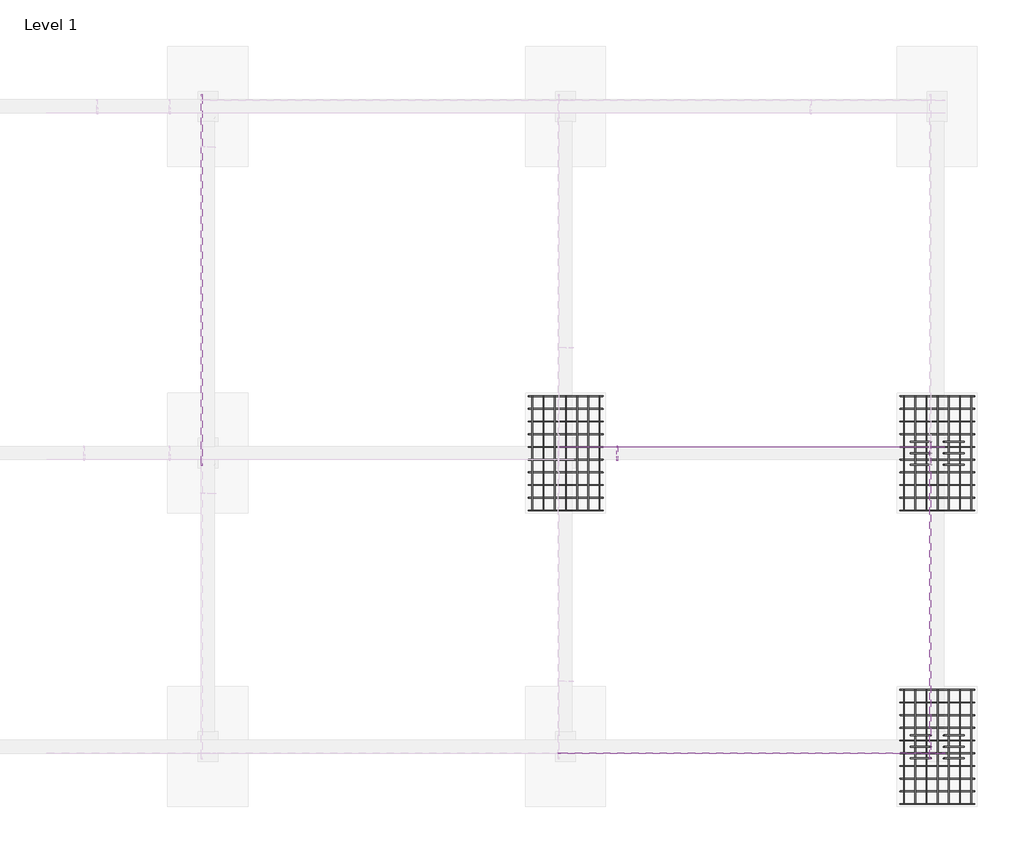
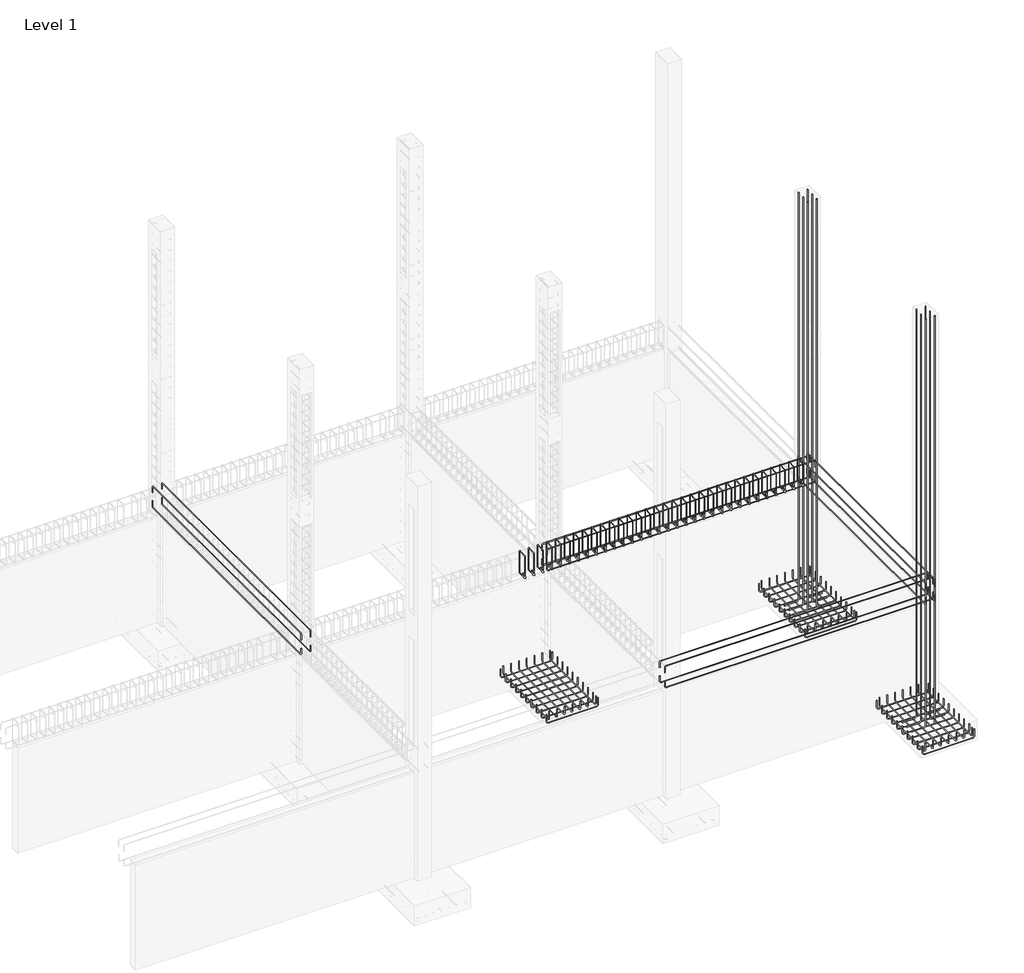
# One storey, part 6 of 8: 19 reinforcing bars.
"""IFC4 building model written with IfcOpenShell, lengths in millimetres."""

from ifc_helpers import new_model, si_unit, point, frame, origin, place, context, project, spatial, polyline, circle_curve, trimmed, segment, composite_curve, source, transform, mapped, element, save
from ifc_brep_helpers import swept_disk

model = new_model("IFC4")

# Units and contexts
model_context = context("Model", 3, world=origin())
ifc_project = project(units=[si_unit("LENGTHUNIT", "METRE", prefix="MILLI")], contexts=[model_context])

# Site, building, storey
site = spatial("IfcSite", under=ifc_project)
building = spatial("IfcBuilding", under=site)
storey = spatial("IfcBuildingStorey", under=building, Name="Level 1", Elevation=0.0)

# Reinforcing bars
placement = place(None, origin())
reinforcing_bar_shape = source(origin(), model_context, "Body", "SolidModel", [
    swept_disk(composite_curve([segment(polyline([(-3147.528716, 3219.1306965, 2643.0183362), (-3147.528716, 3219.1306965, 2528.7183362)]), True, "CONTINUOUS"), segment(trimmed(circle_curve(frame((-3182.072716, 3219.1306965, 2528.7183362), z_axis=(0.0, 1.0, 0.0), x_axis=(34.544000000000324, 0.0, 0.0)), 34.544), [point((-3147.528716, 3219.1306965, 2528.7183362))], [point((-3182.072716, 3219.1306965, 2494.1743362))], True, "CARTESIAN"), True, "CONTINUOUS"), segment(polyline([(-3182.072716, 3219.1306965, 2494.1743362), (-8989.4602157, 3219.1306965, 2494.1743362)]), True, "CONTINUOUS"), segment(trimmed(circle_curve(frame((-8989.4602157, 3219.1306965, 2528.7183362), z_axis=(0.0, 1.0, 0.0), x_axis=(0.0, 0.0, -34.54399999999987)), 34.544), [point((-8989.4602157, 3219.1306965, 2494.1743362))], [point((-9024.0042157, 3219.1306965, 2528.7183362))], True, "CARTESIAN"), True, "CONTINUOUS"), segment(polyline([(-9024.0042157, 3219.1306965, 2528.7183362), (-9024.0042157, 3219.1306965, 2643.0183362)]), True, "CONTINUOUS")], self_intersect=False), 5.969),
])
element("IfcReinforcingBar", 1, at=placement, inside=storey, context=model_context, shape_type="MappedRepresentation", body=[
    mapped(reinforcing_bar_shape, transform((0.0, 0.0, 0.0), x_axis=(1.0, 0.0, 0.0), y_axis=(0.0, 1.0, 0.0), z_axis=(0.0, 0.0, 1.0))),
    mapped(reinforcing_bar_shape, transform((0.0, -193.2513276, 0.0), x_axis=(1.0, 0.0, 0.0), y_axis=(0.0, 1.0, 0.0), z_axis=(0.0, 0.0, 1.0))),
])
reinforcing_bar_2_shape = source(origin(), model_context, "Body", "SolidModel", [
    swept_disk(composite_curve([segment(polyline([(-9024.0042157, 3219.1306965, 2843.3816638), (-9024.0042157, 3219.1306965, 2957.6816638)]), True, "CONTINUOUS"), segment(trimmed(circle_curve(frame((-8989.4602157, 3219.1306965, 2957.6816638), z_axis=(0.0, 1.0, 0.0), x_axis=(-34.54399999999987, 0.0, 0.0)), 34.544), [point((-9024.0042157, 3219.1306965, 2957.6816638))], [point((-8989.4602157, 3219.1306965, 2992.2256638))], True, "CARTESIAN"), True, "CONTINUOUS"), segment(polyline([(-8989.4602157, 3219.1306965, 2992.2256638), (-3182.072716, 3219.1306965, 2992.2256638)]), True, "CONTINUOUS"), segment(trimmed(circle_curve(frame((-3182.072716, 3219.1306965, 2957.6816638), z_axis=(0.0, 1.0, 0.0), x_axis=(0.0, 0.0, 34.54399999999987)), 34.544), [point((-3182.072716, 3219.1306965, 2992.2256638))], [point((-3147.528716, 3219.1306965, 2957.6816638))], True, "CARTESIAN"), True, "CONTINUOUS"), segment(polyline([(-3147.528716, 3219.1306965, 2957.6816638), (-3147.528716, 3219.1306965, 2843.3816638)]), True, "CONTINUOUS")], self_intersect=False), 5.969),
])
element("IfcReinforcingBar", 2, at=placement, inside=storey, context=model_context, shape_type="MappedRepresentation", body=[
    mapped(reinforcing_bar_2_shape, transform((0.0, 0.0, 0.0), x_axis=(1.0, 0.0, 0.0), y_axis=(0.0, 1.0, 0.0), z_axis=(0.0, 0.0, 1.0))),
    mapped(reinforcing_bar_2_shape, transform((0.0, -193.2513276, 0.0), x_axis=(1.0, 0.0, 0.0), y_axis=(0.0, 1.0, 0.0), z_axis=(0.0, 0.0, 1.0))),
])
reinforcing_bar_3_shape = source(origin(), model_context, "Body", "SolidModel", [
    swept_disk(composite_curve([segment(polyline([(-3157.434716, 7767.9070829, 9105.9), (-3157.434716, 7767.9070829, -307.9115)]), True, "CONTINUOUS"), segment(trimmed(circle_curve(frame((-3111.333716, 7767.9070829, -307.9115), z_axis=(0.0, -1.0, 0.0), x_axis=(-46.10100000000011, 0.0, 0.0)), 46.101), [point((-3157.434716, 7767.9070829, -307.9115))], [point((-3111.333716, 7767.9070829, -354.0125))], True, "CARTESIAN"), True, "CONTINUOUS"), segment(polyline([(-3111.333716, 7767.9070829, -354.0125), (-2844.760716, 7767.9070829, -354.0125)]), True, "CONTINUOUS")], self_intersect=False), 8.001),
])
element("IfcReinforcingBar", 3, at=placement, inside=storey, context=model_context, shape_type="MappedRepresentation", body=[
    mapped(reinforcing_bar_3_shape, transform((0.0, 0.0, 0.0), x_axis=(1.0, 0.0, 0.0), y_axis=(0.0, 1.0, 0.0), z_axis=(0.0, 0.0, 1.0))),
    mapped(reinforcing_bar_3_shape, transform((0.0, -174.625, 0.0), x_axis=(1.0, 0.0, 0.0), y_axis=(0.0, 1.0, 0.0), z_axis=(0.0, 0.0, 1.0))),
    mapped(reinforcing_bar_3_shape, transform((0.0, -349.25, 0.0), x_axis=(1.0, 0.0, 0.0), y_axis=(0.0, 1.0, 0.0), z_axis=(0.0, 0.0, 1.0))),
])
reinforcing_bar_4_shape = source(origin(), model_context, "Body", "SolidModel", [
    swept_disk(composite_curve([segment(polyline([(-3666.958716, 7767.9070829, -354.0125), (-3400.385716, 7767.9070829, -354.0125)]), True, "CONTINUOUS"), segment(trimmed(circle_curve(frame((-3400.385716, 7767.9070829, -307.9115), z_axis=(0.0, -1.0, 0.0), x_axis=(0.0, 0.0, -46.101)), 46.101), [point((-3400.385716, 7767.9070829, -354.0125))], [point((-3354.284716, 7767.9070829, -307.9115))], True, "CARTESIAN"), True, "CONTINUOUS"), segment(polyline([(-3354.284716, 7767.9070829, -307.9115), (-3354.284716, 7767.9070829, 9105.9)]), True, "CONTINUOUS")], self_intersect=False), 8.001),
])
element("IfcReinforcingBar", 4, at=placement, inside=storey, context=model_context, shape_type="MappedRepresentation", body=[
    mapped(reinforcing_bar_4_shape, transform((0.0, 0.0, 0.0), x_axis=(1.0, 0.0, 0.0), y_axis=(0.0, 1.0, 0.0), z_axis=(0.0, 0.0, 1.0))),
    mapped(reinforcing_bar_4_shape, transform((0.0, -174.625, 0.0), x_axis=(1.0, 0.0, 0.0), y_axis=(0.0, 1.0, 0.0), z_axis=(0.0, 0.0, 1.0))),
    mapped(reinforcing_bar_4_shape, transform((0.0, -349.25, 0.0), x_axis=(1.0, 0.0, 0.0), y_axis=(0.0, 1.0, 0.0), z_axis=(0.0, 0.0, 1.0))),
])
reinforcing_bar_5_shape = source(origin(), model_context, "Body", "SolidModel", [
    swept_disk(composite_curve([segment(polyline([(-3157.434716, 3297.1300327, 9105.9), (-3157.434716, 3297.1300327, -307.9115)]), True, "CONTINUOUS"), segment(trimmed(circle_curve(frame((-3111.333716, 3297.1300327, -307.9115), z_axis=(0.0, -1.0, 0.0), x_axis=(-46.10100000000011, 0.0, 0.0)), 46.101), [point((-3157.434716, 3297.1300327, -307.9115))], [point((-3111.333716, 3297.1300327, -354.0125))], True, "CARTESIAN"), True, "CONTINUOUS"), segment(polyline([(-3111.333716, 3297.1300327, -354.0125), (-2844.760716, 3297.1300327, -354.0125)]), True, "CONTINUOUS")], self_intersect=False), 8.001),
])
element("IfcReinforcingBar", 5, at=placement, inside=storey, context=model_context, shape_type="MappedRepresentation", body=[
    mapped(reinforcing_bar_5_shape, transform((0.0, 0.0, 0.0), x_axis=(1.0, 0.0, 0.0), y_axis=(0.0, 1.0, 0.0), z_axis=(0.0, 0.0, 1.0))),
    mapped(reinforcing_bar_5_shape, transform((0.0, -174.625, 0.0), x_axis=(1.0, 0.0, 0.0), y_axis=(0.0, 1.0, 0.0), z_axis=(0.0, 0.0, 1.0))),
    mapped(reinforcing_bar_5_shape, transform((0.0, -349.25, 0.0), x_axis=(1.0, 0.0, 0.0), y_axis=(0.0, 1.0, 0.0), z_axis=(0.0, 0.0, 1.0))),
])
reinforcing_bar_6_shape = source(origin(), model_context, "Body", "SolidModel", [
    swept_disk(composite_curve([segment(polyline([(-3666.958716, 3297.1300327, -354.0125), (-3400.385716, 3297.1300327, -354.0125)]), True, "CONTINUOUS"), segment(trimmed(circle_curve(frame((-3400.385716, 3297.1300327, -307.9115), z_axis=(0.0, -1.0, 0.0), x_axis=(0.0, 0.0, -46.101)), 46.101), [point((-3400.385716, 3297.1300327, -354.0125))], [point((-3354.284716, 3297.1300327, -307.9115))], True, "CARTESIAN"), True, "CONTINUOUS"), segment(polyline([(-3354.284716, 3297.1300327, -307.9115), (-3354.284716, 3297.1300327, 9105.9)]), True, "CONTINUOUS")], self_intersect=False), 8.001),
])
element("IfcReinforcingBar", 6, at=placement, inside=storey, context=model_context, shape_type="MappedRepresentation", body=[
    mapped(reinforcing_bar_6_shape, transform((0.0, 0.0, 0.0), x_axis=(1.0, 0.0, 0.0), y_axis=(0.0, 1.0, 0.0), z_axis=(0.0, 0.0, 1.0))),
    mapped(reinforcing_bar_6_shape, transform((0.0, -174.625, 0.0), x_axis=(1.0, 0.0, 0.0), y_axis=(0.0, 1.0, 0.0), z_axis=(0.0, 0.0, 1.0))),
    mapped(reinforcing_bar_6_shape, transform((0.0, -349.25, 0.0), x_axis=(1.0, 0.0, 0.0), y_axis=(0.0, 1.0, 0.0), z_axis=(0.0, 0.0, 1.0))),
])
reinforcing_bar_7_shape = source(origin(), model_context, "Body", "SolidModel", [
    swept_disk(composite_curve([segment(polyline([(-2690.328716, 8463.6130829, -216.662), (-2690.328716, 8463.6130829, -369.062)]), True, "CONTINUOUS"), segment(trimmed(circle_curve(frame((-2734.397716, 8463.6130829, -369.062), z_axis=(0.0, 1.0, 0.0), x_axis=(44.06899999999996, 0.0, 0.0)), 44.069), [point((-2690.328716, 8463.6130829, -369.062))], [point((-2734.397716, 8463.6130829, -413.131))], True, "CARTESIAN"), True, "CONTINUOUS"), segment(polyline([(-2734.397716, 8463.6130829, -413.131), (-3777.321716, 8463.6130829, -413.131)]), True, "CONTINUOUS"), segment(trimmed(circle_curve(frame((-3777.321716, 8463.6130829, -369.062), z_axis=(0.0, 1.0, 0.0), x_axis=(0.0, 0.0, -44.06899999999996)), 44.069), [point((-3777.321716, 8463.6130829, -413.131))], [point((-3821.390716, 8463.6130829, -369.062))], True, "CARTESIAN"), True, "CONTINUOUS"), segment(polyline([(-3821.390716, 8463.6130829, -369.062), (-3821.390716, 8463.6130829, -216.662)]), True, "CONTINUOUS")], self_intersect=False), 5.969),
])
element("IfcReinforcingBar", 7, at=placement, inside=storey, context=model_context, shape_type="MappedRepresentation", body=[
    mapped(reinforcing_bar_7_shape, transform((0.0, 0.0, 0.0), x_axis=(1.0, 0.0, 0.0), y_axis=(0.0, 1.0, 0.0), z_axis=(0.0, 0.0, 1.0))),
    mapped(reinforcing_bar_7_shape, transform((0.0, -193.4068889, 0.0), x_axis=(1.0, 0.0, 0.0), y_axis=(0.0, 1.0, 0.0), z_axis=(0.0, 0.0, 1.0))),
    mapped(reinforcing_bar_7_shape, transform((0.0, -386.8137778, 0.0), x_axis=(1.0, 0.0, 0.0), y_axis=(0.0, 1.0, 0.0), z_axis=(0.0, 0.0, 1.0))),
    mapped(reinforcing_bar_7_shape, transform((0.0, -580.2206667, 0.0), x_axis=(1.0, 0.0, 0.0), y_axis=(0.0, 1.0, 0.0), z_axis=(0.0, 0.0, 1.0))),
    mapped(reinforcing_bar_7_shape, transform((0.0, -773.6275556, 0.0), x_axis=(1.0, 0.0, 0.0), y_axis=(0.0, 1.0, 0.0), z_axis=(0.0, 0.0, 1.0))),
    mapped(reinforcing_bar_7_shape, transform((0.0, -967.0344444, 0.0), x_axis=(1.0, 0.0, 0.0), y_axis=(0.0, 1.0, 0.0), z_axis=(0.0, 0.0, 1.0))),
    mapped(reinforcing_bar_7_shape, transform((0.0, -1160.4413333, 0.0), x_axis=(1.0, 0.0, 0.0), y_axis=(0.0, 1.0, 0.0), z_axis=(0.0, 0.0, 1.0))),
    mapped(reinforcing_bar_7_shape, transform((0.0, -1353.8482222, 0.0), x_axis=(1.0, 0.0, 0.0), y_axis=(0.0, 1.0, 0.0), z_axis=(0.0, 0.0, 1.0))),
    mapped(reinforcing_bar_7_shape, transform((0.0, -1547.2551111, 0.0), x_axis=(1.0, 0.0, 0.0), y_axis=(0.0, 1.0, 0.0), z_axis=(0.0, 0.0, 1.0))),
    mapped(reinforcing_bar_7_shape, transform((0.0, -1740.662, 0.0), x_axis=(1.0, 0.0, 0.0), y_axis=(0.0, 1.0, 0.0), z_axis=(0.0, 0.0, 1.0))),
])
reinforcing_bar_8_shape = source(origin(), model_context, "Body", "SolidModel", [
    swept_disk(composite_curve([segment(polyline([(-3763.859716, 8463.6130829, -165.481), (-3763.859716, 8463.6130829, -317.881)]), True, "CONTINUOUS"), segment(trimmed(circle_curve(frame((-3763.859716, 8419.5440829, -317.881), z_axis=(-1.0, 0.0, 0.0), x_axis=(0.0, 44.068999999999505, 0.0)), 44.069), [point((-3763.859716, 8463.6130829, -317.881))], [point((-3763.859716, 8419.5440829, -361.95))], True, "CARTESIAN"), True, "CONTINUOUS"), segment(polyline([(-3763.859716, 8419.5440829, -361.95), (-3763.859716, 6767.0200829, -361.95)]), True, "CONTINUOUS"), segment(trimmed(circle_curve(frame((-3763.859716, 6767.0200829, -317.881), z_axis=(-1.0, 0.0, 0.0), x_axis=(0.0, 0.0, -44.06900000000002)), 44.069), [point((-3763.859716, 6767.0200829, -361.95))], [point((-3763.859716, 6722.9510829, -317.881))], True, "CARTESIAN"), True, "CONTINUOUS"), segment(polyline([(-3763.859716, 6722.9510829, -317.881), (-3763.859716, 6722.9510829, -165.481)]), True, "CONTINUOUS")], self_intersect=False), 5.969),
])
element("IfcReinforcingBar", 8, at=placement, inside=storey, context=model_context, shape_type="MappedRepresentation", body=[
    mapped(reinforcing_bar_8_shape, transform((0.0, 0.0, 0.0), x_axis=(1.0, 0.0, 0.0), y_axis=(0.0, 1.0, 0.0), z_axis=(0.0, 0.0, 1.0))),
    mapped(reinforcing_bar_8_shape, transform((170.5954914, 0.0, 0.0), x_axis=(1.0, 0.0, 0.0), y_axis=(0.0, 1.0, 0.0), z_axis=(0.0, 0.0, 1.0))),
    mapped(reinforcing_bar_8_shape, transform((341.1909829, 0.0, 0.0), x_axis=(1.0, 0.0, 0.0), y_axis=(0.0, 1.0, 0.0), z_axis=(0.0, 0.0, 1.0))),
    mapped(reinforcing_bar_8_shape, transform((511.7864743, 0.0, 0.0), x_axis=(1.0, 0.0, 0.0), y_axis=(0.0, 1.0, 0.0), z_axis=(0.0, 0.0, 1.0))),
    mapped(reinforcing_bar_8_shape, transform((682.3819658, 0.0, 0.0), x_axis=(1.0, 0.0, 0.0), y_axis=(0.0, 1.0, 0.0), z_axis=(0.0, 0.0, 1.0))),
    mapped(reinforcing_bar_8_shape, transform((852.9774572, 0.0, 0.0), x_axis=(1.0, 0.0, 0.0), y_axis=(0.0, 1.0, 0.0), z_axis=(0.0, 0.0, 1.0))),
    mapped(reinforcing_bar_8_shape, transform((1023.5729487, 0.0, 0.0), x_axis=(1.0, 0.0, 0.0), y_axis=(0.0, 1.0, 0.0), z_axis=(0.0, 0.0, 1.0))),
])
reinforcing_bar_9_shape = source(origin(), model_context, "Body", "SolidModel", [
    swept_disk(composite_curve([segment(polyline([(-8350.1422157, 8463.6130829, -216.662), (-8350.1422157, 8463.6130829, -369.062)]), True, "CONTINUOUS"), segment(trimmed(circle_curve(frame((-8394.2112157, 8463.6130829, -369.062), z_axis=(0.0, 1.0, 0.0), x_axis=(44.068999999999505, 0.0, 0.0)), 44.069), [point((-8350.1422157, 8463.6130829, -369.062))], [point((-8394.2112157, 8463.6130829, -413.131))], True, "CARTESIAN"), True, "CONTINUOUS"), segment(polyline([(-8394.2112157, 8463.6130829, -413.131), (-9437.1352157, 8463.6130829, -413.131)]), True, "CONTINUOUS"), segment(trimmed(circle_curve(frame((-9437.1352157, 8463.6130829, -369.062), z_axis=(0.0, 1.0, 0.0), x_axis=(0.0, 0.0, -44.06899999999996)), 44.069), [point((-9437.1352157, 8463.6130829, -413.131))], [point((-9481.2042157, 8463.6130829, -369.062))], True, "CARTESIAN"), True, "CONTINUOUS"), segment(polyline([(-9481.2042157, 8463.6130829, -369.062), (-9481.2042157, 8463.6130829, -216.662)]), True, "CONTINUOUS")], self_intersect=False), 5.969),
])
element("IfcReinforcingBar", 9, at=placement, inside=storey, context=model_context, shape_type="MappedRepresentation", body=[
    mapped(reinforcing_bar_9_shape, transform((0.0, 0.0, 0.0), x_axis=(1.0, 0.0, 0.0), y_axis=(0.0, 1.0, 0.0), z_axis=(0.0, 0.0, 1.0))),
    mapped(reinforcing_bar_9_shape, transform((0.0, -193.4068889, 0.0), x_axis=(1.0, 0.0, 0.0), y_axis=(0.0, 1.0, 0.0), z_axis=(0.0, 0.0, 1.0))),
    mapped(reinforcing_bar_9_shape, transform((0.0, -386.8137778, 0.0), x_axis=(1.0, 0.0, 0.0), y_axis=(0.0, 1.0, 0.0), z_axis=(0.0, 0.0, 1.0))),
    mapped(reinforcing_bar_9_shape, transform((0.0, -580.2206667, 0.0), x_axis=(1.0, 0.0, 0.0), y_axis=(0.0, 1.0, 0.0), z_axis=(0.0, 0.0, 1.0))),
    mapped(reinforcing_bar_9_shape, transform((0.0, -773.6275556, 0.0), x_axis=(1.0, 0.0, 0.0), y_axis=(0.0, 1.0, 0.0), z_axis=(0.0, 0.0, 1.0))),
    mapped(reinforcing_bar_9_shape, transform((0.0, -967.0344444, 0.0), x_axis=(1.0, 0.0, 0.0), y_axis=(0.0, 1.0, 0.0), z_axis=(0.0, 0.0, 1.0))),
    mapped(reinforcing_bar_9_shape, transform((0.0, -1160.4413333, 0.0), x_axis=(1.0, 0.0, 0.0), y_axis=(0.0, 1.0, 0.0), z_axis=(0.0, 0.0, 1.0))),
    mapped(reinforcing_bar_9_shape, transform((0.0, -1353.8482222, 0.0), x_axis=(1.0, 0.0, 0.0), y_axis=(0.0, 1.0, 0.0), z_axis=(0.0, 0.0, 1.0))),
    mapped(reinforcing_bar_9_shape, transform((0.0, -1547.2551111, 0.0), x_axis=(1.0, 0.0, 0.0), y_axis=(0.0, 1.0, 0.0), z_axis=(0.0, 0.0, 1.0))),
    mapped(reinforcing_bar_9_shape, transform((0.0, -1740.662, 0.0), x_axis=(1.0, 0.0, 0.0), y_axis=(0.0, 1.0, 0.0), z_axis=(0.0, 0.0, 1.0))),
])
reinforcing_bar_10_shape = source(origin(), model_context, "Body", "SolidModel", [
    swept_disk(composite_curve([segment(polyline([(-9423.6732157, 8463.6130829, -165.481), (-9423.6732157, 8463.6130829, -317.881)]), True, "CONTINUOUS"), segment(trimmed(circle_curve(frame((-9423.6732157, 8419.5440829, -317.881), z_axis=(-1.0, 0.0, 0.0), x_axis=(0.0, 44.068999999999505, 0.0)), 44.069), [point((-9423.6732157, 8463.6130829, -317.881))], [point((-9423.6732157, 8419.5440829, -361.95))], True, "CARTESIAN"), True, "CONTINUOUS"), segment(polyline([(-9423.6732157, 8419.5440829, -361.95), (-9423.6732157, 6767.0200829, -361.95)]), True, "CONTINUOUS"), segment(trimmed(circle_curve(frame((-9423.6732157, 6767.0200829, -317.881), z_axis=(-1.0, 0.0, 0.0), x_axis=(0.0, 0.0, -44.06900000000002)), 44.069), [point((-9423.6732157, 6767.0200829, -361.95))], [point((-9423.6732157, 6722.9510829, -317.881))], True, "CARTESIAN"), True, "CONTINUOUS"), segment(polyline([(-9423.6732157, 6722.9510829, -317.881), (-9423.6732157, 6722.9510829, -165.481)]), True, "CONTINUOUS")], self_intersect=False), 5.969),
])
element("IfcReinforcingBar", 10, at=placement, inside=storey, context=model_context, shape_type="MappedRepresentation", body=[
    mapped(reinforcing_bar_10_shape, transform((0.0, 0.0, 0.0), x_axis=(1.0, 0.0, 0.0), y_axis=(0.0, 1.0, 0.0), z_axis=(0.0, 0.0, 1.0))),
    mapped(reinforcing_bar_10_shape, transform((170.5954914, 0.0, 0.0), x_axis=(1.0, 0.0, 0.0), y_axis=(0.0, 1.0, 0.0), z_axis=(0.0, 0.0, 1.0))),
    mapped(reinforcing_bar_10_shape, transform((341.1909829, 0.0, 0.0), x_axis=(1.0, 0.0, 0.0), y_axis=(0.0, 1.0, 0.0), z_axis=(0.0, 0.0, 1.0))),
    mapped(reinforcing_bar_10_shape, transform((511.7864743, 0.0, 0.0), x_axis=(1.0, 0.0, 0.0), y_axis=(0.0, 1.0, 0.0), z_axis=(0.0, 0.0, 1.0))),
    mapped(reinforcing_bar_10_shape, transform((682.3819658, 0.0, 0.0), x_axis=(1.0, 0.0, 0.0), y_axis=(0.0, 1.0, 0.0), z_axis=(0.0, 0.0, 1.0))),
    mapped(reinforcing_bar_10_shape, transform((852.9774572, 0.0, 0.0), x_axis=(1.0, 0.0, 0.0), y_axis=(0.0, 1.0, 0.0), z_axis=(0.0, 0.0, 1.0))),
    mapped(reinforcing_bar_10_shape, transform((1023.5729487, 0.0, 0.0), x_axis=(1.0, 0.0, 0.0), y_axis=(0.0, 1.0, 0.0), z_axis=(0.0, 0.0, 1.0))),
])
reinforcing_bar_11_shape = source(origin(), model_context, "Body", "SolidModel", [
    swept_disk(composite_curve([segment(polyline([(-2690.328716, 3992.8360327, -216.662), (-2690.328716, 3992.8360327, -369.062)]), True, "CONTINUOUS"), segment(trimmed(circle_curve(frame((-2734.397716, 3992.8360327, -369.062), z_axis=(0.0, 1.0, 0.0), x_axis=(44.06899999999996, 0.0, 0.0)), 44.069), [point((-2690.328716, 3992.8360327, -369.062))], [point((-2734.397716, 3992.8360327, -413.131))], True, "CARTESIAN"), True, "CONTINUOUS"), segment(polyline([(-2734.397716, 3992.8360327, -413.131), (-3777.321716, 3992.8360327, -413.131)]), True, "CONTINUOUS"), segment(trimmed(circle_curve(frame((-3777.321716, 3992.8360327, -369.062), z_axis=(0.0, 1.0, 0.0), x_axis=(0.0, 0.0, -44.06899999999996)), 44.069), [point((-3777.321716, 3992.8360327, -413.131))], [point((-3821.390716, 3992.8360327, -369.062))], True, "CARTESIAN"), True, "CONTINUOUS"), segment(polyline([(-3821.390716, 3992.8360327, -369.062), (-3821.390716, 3992.8360327, -216.662)]), True, "CONTINUOUS")], self_intersect=False), 5.969),
])
element("IfcReinforcingBar", 11, at=placement, inside=storey, context=model_context, shape_type="MappedRepresentation", body=[
    mapped(reinforcing_bar_11_shape, transform((0.0, 0.0, 0.0), x_axis=(1.0, 0.0, 0.0), y_axis=(0.0, 1.0, 0.0), z_axis=(0.0, 0.0, 1.0))),
    mapped(reinforcing_bar_11_shape, transform((0.0, -193.4068889, 0.0), x_axis=(1.0, 0.0, 0.0), y_axis=(0.0, 1.0, 0.0), z_axis=(0.0, 0.0, 1.0))),
    mapped(reinforcing_bar_11_shape, transform((0.0, -386.8137778, 0.0), x_axis=(1.0, 0.0, 0.0), y_axis=(0.0, 1.0, 0.0), z_axis=(0.0, 0.0, 1.0))),
    mapped(reinforcing_bar_11_shape, transform((0.0, -580.2206667, 0.0), x_axis=(1.0, 0.0, 0.0), y_axis=(0.0, 1.0, 0.0), z_axis=(0.0, 0.0, 1.0))),
    mapped(reinforcing_bar_11_shape, transform((0.0, -773.6275556, 0.0), x_axis=(1.0, 0.0, 0.0), y_axis=(0.0, 1.0, 0.0), z_axis=(0.0, 0.0, 1.0))),
    mapped(reinforcing_bar_11_shape, transform((0.0, -967.0344444, 0.0), x_axis=(1.0, 0.0, 0.0), y_axis=(0.0, 1.0, 0.0), z_axis=(0.0, 0.0, 1.0))),
    mapped(reinforcing_bar_11_shape, transform((0.0, -1160.4413333, 0.0), x_axis=(1.0, 0.0, 0.0), y_axis=(0.0, 1.0, 0.0), z_axis=(0.0, 0.0, 1.0))),
    mapped(reinforcing_bar_11_shape, transform((0.0, -1353.8482222, 0.0), x_axis=(1.0, 0.0, 0.0), y_axis=(0.0, 1.0, 0.0), z_axis=(0.0, 0.0, 1.0))),
    mapped(reinforcing_bar_11_shape, transform((0.0, -1547.2551111, 0.0), x_axis=(1.0, 0.0, 0.0), y_axis=(0.0, 1.0, 0.0), z_axis=(0.0, 0.0, 1.0))),
    mapped(reinforcing_bar_11_shape, transform((0.0, -1740.662, 0.0), x_axis=(1.0, 0.0, 0.0), y_axis=(0.0, 1.0, 0.0), z_axis=(0.0, 0.0, 1.0))),
])
reinforcing_bar_12_shape = source(origin(), model_context, "Body", "SolidModel", [
    swept_disk(composite_curve([segment(polyline([(-3763.859716, 3992.8360327, -165.481), (-3763.859716, 3992.8360327, -317.881)]), True, "CONTINUOUS"), segment(trimmed(circle_curve(frame((-3763.859716, 3948.7670327, -317.881), z_axis=(-1.0, 0.0, 0.0), x_axis=(0.0, 44.06899999999996, 0.0)), 44.069), [point((-3763.859716, 3992.8360327, -317.881))], [point((-3763.859716, 3948.7670327, -361.95))], True, "CARTESIAN"), True, "CONTINUOUS"), segment(polyline([(-3763.859716, 3948.7670327, -361.95), (-3763.859716, 2296.2430327, -361.95)]), True, "CONTINUOUS"), segment(trimmed(circle_curve(frame((-3763.859716, 2296.2430327, -317.881), z_axis=(-1.0, 0.0, 0.0), x_axis=(0.0, 0.0, -44.06900000000002)), 44.069), [point((-3763.859716, 2296.2430327, -361.95))], [point((-3763.859716, 2252.1740327, -317.881))], True, "CARTESIAN"), True, "CONTINUOUS"), segment(polyline([(-3763.859716, 2252.1740327, -317.881), (-3763.859716, 2252.1740327, -165.481)]), True, "CONTINUOUS")], self_intersect=False), 5.969),
])
element("IfcReinforcingBar", 12, at=placement, inside=storey, context=model_context, shape_type="MappedRepresentation", body=[
    mapped(reinforcing_bar_12_shape, transform((0.0, 0.0, 0.0), x_axis=(1.0, 0.0, 0.0), y_axis=(0.0, 1.0, 0.0), z_axis=(0.0, 0.0, 1.0))),
    mapped(reinforcing_bar_12_shape, transform((170.5954914, 0.0, 0.0), x_axis=(1.0, 0.0, 0.0), y_axis=(0.0, 1.0, 0.0), z_axis=(0.0, 0.0, 1.0))),
    mapped(reinforcing_bar_12_shape, transform((341.1909829, 0.0, 0.0), x_axis=(1.0, 0.0, 0.0), y_axis=(0.0, 1.0, 0.0), z_axis=(0.0, 0.0, 1.0))),
    mapped(reinforcing_bar_12_shape, transform((511.7864743, 0.0, 0.0), x_axis=(1.0, 0.0, 0.0), y_axis=(0.0, 1.0, 0.0), z_axis=(0.0, 0.0, 1.0))),
    mapped(reinforcing_bar_12_shape, transform((682.3819658, 0.0, 0.0), x_axis=(1.0, 0.0, 0.0), y_axis=(0.0, 1.0, 0.0), z_axis=(0.0, 0.0, 1.0))),
    mapped(reinforcing_bar_12_shape, transform((852.9774572, 0.0, 0.0), x_axis=(1.0, 0.0, 0.0), y_axis=(0.0, 1.0, 0.0), z_axis=(0.0, 0.0, 1.0))),
    mapped(reinforcing_bar_12_shape, transform((1023.5729487, 0.0, 0.0), x_axis=(1.0, 0.0, 0.0), y_axis=(0.0, 1.0, 0.0), z_axis=(0.0, 0.0, 1.0))),
])
reinforcing_bar_13_shape = source(origin(), model_context, "Body", "SolidModel", [
    swept_disk(composite_curve([segment(polyline([(-9024.0042157, 7496.6564191, 2643.0183362), (-9024.0042157, 7496.6564191, 2528.7183362)]), True, "CONTINUOUS"), segment(trimmed(circle_curve(frame((-8989.4602157, 7496.6564191, 2528.7183362), z_axis=(0.0, -1.0, 0.0), x_axis=(-34.54399999999987, 0.0, 0.0)), 34.544), [point((-9024.0042157, 7496.6564191, 2528.7183362))], [point((-8989.4602157, 7496.6564191, 2494.1743362))], True, "CARTESIAN"), True, "CONTINUOUS"), segment(polyline([(-8989.4602157, 7496.6564191, 2494.1743362), (-3182.072716, 7496.6564191, 2494.1743362)]), True, "CONTINUOUS"), segment(trimmed(circle_curve(frame((-3182.072716, 7496.6564191, 2528.7183362), z_axis=(0.0, -1.0, 0.0), x_axis=(0.0, 0.0, -34.54399999999987)), 34.544), [point((-3182.072716, 7496.6564191, 2494.1743362))], [point((-3147.528716, 7496.6564191, 2528.7183362))], True, "CARTESIAN"), True, "CONTINUOUS"), segment(polyline([(-3147.528716, 7496.6564191, 2528.7183362), (-3147.528716, 7496.6564191, 2643.0183362)]), True, "CONTINUOUS")], self_intersect=False), 5.969),
])
element("IfcReinforcingBar", 13, at=placement, inside=storey, context=model_context, shape_type="MappedRepresentation", body=[
    mapped(reinforcing_bar_13_shape, transform((0.0, 0.0, 0.0), x_axis=(1.0, 0.0, 0.0), y_axis=(0.0, 1.0, 0.0), z_axis=(0.0, 0.0, 1.0))),
    mapped(reinforcing_bar_13_shape, transform((0.0, 193.2513276, 0.0), x_axis=(1.0, 0.0, 0.0), y_axis=(0.0, 1.0, 0.0), z_axis=(0.0, 0.0, 1.0))),
])
reinforcing_bar_14_shape = source(origin(), model_context, "Body", "SolidModel", [
    swept_disk(composite_curve([segment(polyline([(-3147.528716, 7496.6564191, 2843.3816638), (-3147.528716, 7496.6564191, 2957.6816638)]), True, "CONTINUOUS"), segment(trimmed(circle_curve(frame((-3182.072716, 7496.6564191, 2957.6816638), z_axis=(0.0, -1.0, 0.0), x_axis=(34.544000000000324, 0.0, 0.0)), 34.544), [point((-3147.528716, 7496.6564191, 2957.6816638))], [point((-3182.072716, 7496.6564191, 2992.2256638))], True, "CARTESIAN"), True, "CONTINUOUS"), segment(polyline([(-3182.072716, 7496.6564191, 2992.2256638), (-8989.4602157, 7496.6564191, 2992.2256638)]), True, "CONTINUOUS"), segment(trimmed(circle_curve(frame((-8989.4602157, 7496.6564191, 2957.6816638), z_axis=(0.0, -1.0, 0.0), x_axis=(0.0, 0.0, 34.54399999999987)), 34.544), [point((-8989.4602157, 7496.6564191, 2992.2256638))], [point((-9024.0042157, 7496.6564191, 2957.6816638))], True, "CARTESIAN"), True, "CONTINUOUS"), segment(polyline([(-9024.0042157, 7496.6564191, 2957.6816638), (-9024.0042157, 7496.6564191, 2843.3816638)]), True, "CONTINUOUS")], self_intersect=False), 5.969),
])
element("IfcReinforcingBar", 14, at=placement, inside=storey, context=model_context, shape_type="MappedRepresentation", body=[
    mapped(reinforcing_bar_14_shape, transform((0.0, 0.0, 0.0), x_axis=(1.0, 0.0, 0.0), y_axis=(0.0, 1.0, 0.0), z_axis=(0.0, 0.0, 1.0))),
    mapped(reinforcing_bar_14_shape, transform((0.0, 193.2513276, 0.0), x_axis=(1.0, 0.0, 0.0), y_axis=(0.0, 1.0, 0.0), z_axis=(0.0, 0.0, 1.0))),
])
reinforcing_bar_15_shape = source(origin(), model_context, "Body", "SolidModel", [
    swept_disk(composite_curve([segment(polyline([(-9504.1968704, 7546.5160164, 2576.5424606), (-9504.1968704, 7489.6518193, 2519.6782636)]), True, "CONTINUOUS"), segment(trimmed(circle_curve(frame((-9504.1968704, 7505.9060829, 2503.424), z_axis=(1.0, 0.0, 0.0), x_axis=(0.0, -16.25426359999983, 16.25426359999983)), 22.987), [point((-9504.1968704, 7489.6518193, 2519.6782636))], [point((-9504.1968704, 7505.9060829, 2480.437))], True, "CARTESIAN"), True, "CONTINUOUS"), segment(polyline([(-9504.1968704, 7505.9060829, 2480.437), (-9504.1968704, 7680.6580829, 2480.437)]), True, "CONTINUOUS"), segment(trimmed(circle_curve(frame((-9504.1968704, 7680.6580829, 2503.424), z_axis=(1.0, 0.0, 0.0), x_axis=(0.0, 0.0, -22.98700000000008)), 22.987), [point((-9504.1968704, 7680.6580829, 2480.437))], [point((-9504.1968704, 7703.6450829, 2503.424))], True, "CARTESIAN"), True, "CONTINUOUS"), segment(polyline([(-9504.1968704, 7703.6450829, 2503.424), (-9504.1968704, 7703.6450829, 2982.976)]), True, "CONTINUOUS"), segment(trimmed(circle_curve(frame((-9505.0163687, 7680.6726953, 2982.976), z_axis=(0.999364318494848, -0.03565051078635566, 0.0), x_axis=(0.8194983000012144, 22.97238759999982, 0.0)), 22.987), [point((-9504.1968704, 7703.6450829, 2982.976))], [point((-9505.0163687, 7680.6726953, 3005.963))], True, "CARTESIAN"), True, "CONTINUOUS"), segment(polyline([(-9505.0163687, 7680.6726953, 3005.963), (-9511.2513721, 7505.8914705, 3005.963)]), True, "CONTINUOUS"), segment(trimmed(circle_curve(frame((-9511.2513721, 7505.8914705, 2982.976), z_axis=(0.999364318494848, -0.03565051078635566, 0.0), x_axis=(0.0, 0.0, 22.98700000000008)), 22.987), [point((-9511.2513721, 7505.8914705, 3005.963))], [point((-9512.0708704, 7482.9190829, 2982.976))], True, "CARTESIAN"), True, "CONTINUOUS"), segment(polyline([(-9512.0708704, 7482.9190829, 2982.976), (-9512.0708704, 7482.9190829, 2503.424)]), True, "CONTINUOUS"), segment(trimmed(circle_curve(frame((-9512.0708704, 7505.9060829, 2503.424), z_axis=(1.0, 0.0, 0.0), x_axis=(0.0, -22.98700000000008, 0.0)), 22.987), [point((-9512.0708704, 7482.9190829, 2503.424))], [point((-9512.0708704, 7522.1603465, 2487.1697364))], True, "CARTESIAN"), True, "CONTINUOUS"), segment(polyline([(-9512.0708704, 7522.1603465, 2487.1697364), (-9512.0708704, 7579.0245435, 2544.0339335)]), True, "CONTINUOUS")], self_intersect=False), 3.937),
])
element("IfcReinforcingBar", 15, at=placement, inside=storey, context=model_context, shape_type="MappedRepresentation", body=[
    mapped(reinforcing_bar_15_shape, transform((0.0, 0.0, 0.0), x_axis=(1.0, 0.0, 0.0), y_axis=(0.0, 1.0, 0.0), z_axis=(0.0, 0.0, 1.0))),
    mapped(reinforcing_bar_15_shape, transform((196.516134, 0.0, 0.0), x_axis=(1.0, 0.0, 0.0), y_axis=(0.0, 1.0, 0.0), z_axis=(0.0, 0.0, 1.0))),
    mapped(reinforcing_bar_15_shape, transform((393.032268, 0.0, 0.0), x_axis=(1.0, 0.0, 0.0), y_axis=(0.0, 1.0, 0.0), z_axis=(0.0, 0.0, 1.0))),
    mapped(reinforcing_bar_15_shape, transform((589.548402, 0.0, 0.0), x_axis=(1.0, 0.0, 0.0), y_axis=(0.0, 1.0, 0.0), z_axis=(0.0, 0.0, 1.0))),
    mapped(reinforcing_bar_15_shape, transform((786.0645361, 0.0, 0.0), x_axis=(1.0, 0.0, 0.0), y_axis=(0.0, 1.0, 0.0), z_axis=(0.0, 0.0, 1.0))),
    mapped(reinforcing_bar_15_shape, transform((982.5806701, 0.0, 0.0), x_axis=(1.0, 0.0, 0.0), y_axis=(0.0, 1.0, 0.0), z_axis=(0.0, 0.0, 1.0))),
    mapped(reinforcing_bar_15_shape, transform((1179.0968041, 0.0, 0.0), x_axis=(1.0, 0.0, 0.0), y_axis=(0.0, 1.0, 0.0), z_axis=(0.0, 0.0, 1.0))),
    mapped(reinforcing_bar_15_shape, transform((1375.6129381, 0.0, 0.0), x_axis=(1.0, 0.0, 0.0), y_axis=(0.0, 1.0, 0.0), z_axis=(0.0, 0.0, 1.0))),
    mapped(reinforcing_bar_15_shape, transform((1572.1290721, 0.0, 0.0), x_axis=(1.0, 0.0, 0.0), y_axis=(0.0, 1.0, 0.0), z_axis=(0.0, 0.0, 1.0))),
    mapped(reinforcing_bar_15_shape, transform((1768.6452061, 0.0, 0.0), x_axis=(1.0, 0.0, 0.0), y_axis=(0.0, 1.0, 0.0), z_axis=(0.0, 0.0, 1.0))),
    mapped(reinforcing_bar_15_shape, transform((1965.1613401, 0.0, 0.0), x_axis=(1.0, 0.0, 0.0), y_axis=(0.0, 1.0, 0.0), z_axis=(0.0, 0.0, 1.0))),
    mapped(reinforcing_bar_15_shape, transform((2161.6774741, 0.0, 0.0), x_axis=(1.0, 0.0, 0.0), y_axis=(0.0, 1.0, 0.0), z_axis=(0.0, 0.0, 1.0))),
    mapped(reinforcing_bar_15_shape, transform((2358.1936082, 0.0, 0.0), x_axis=(1.0, 0.0, 0.0), y_axis=(0.0, 1.0, 0.0), z_axis=(0.0, 0.0, 1.0))),
    mapped(reinforcing_bar_15_shape, transform((2554.7097422, 0.0, 0.0), x_axis=(1.0, 0.0, 0.0), y_axis=(0.0, 1.0, 0.0), z_axis=(0.0, 0.0, 1.0))),
    mapped(reinforcing_bar_15_shape, transform((2751.2258762, 0.0, 0.0), x_axis=(1.0, 0.0, 0.0), y_axis=(0.0, 1.0, 0.0), z_axis=(0.0, 0.0, 1.0))),
    mapped(reinforcing_bar_15_shape, transform((2947.7420102, 0.0, 0.0), x_axis=(1.0, 0.0, 0.0), y_axis=(0.0, 1.0, 0.0), z_axis=(0.0, 0.0, 1.0))),
    mapped(reinforcing_bar_15_shape, transform((3144.2581442, 0.0, 0.0), x_axis=(1.0, 0.0, 0.0), y_axis=(0.0, 1.0, 0.0), z_axis=(0.0, 0.0, 1.0))),
    mapped(reinforcing_bar_15_shape, transform((3340.7742782, 0.0, 0.0), x_axis=(1.0, 0.0, 0.0), y_axis=(0.0, 1.0, 0.0), z_axis=(0.0, 0.0, 1.0))),
    mapped(reinforcing_bar_15_shape, transform((3537.2904122, 0.0, 0.0), x_axis=(1.0, 0.0, 0.0), y_axis=(0.0, 1.0, 0.0), z_axis=(0.0, 0.0, 1.0))),
    mapped(reinforcing_bar_15_shape, transform((3733.8065462, 0.0, 0.0), x_axis=(1.0, 0.0, 0.0), y_axis=(0.0, 1.0, 0.0), z_axis=(0.0, 0.0, 1.0))),
    mapped(reinforcing_bar_15_shape, transform((3930.3226803, 0.0, 0.0), x_axis=(1.0, 0.0, 0.0), y_axis=(0.0, 1.0, 0.0), z_axis=(0.0, 0.0, 1.0))),
    mapped(reinforcing_bar_15_shape, transform((4126.8388143, 0.0, 0.0), x_axis=(1.0, 0.0, 0.0), y_axis=(0.0, 1.0, 0.0), z_axis=(0.0, 0.0, 1.0))),
    mapped(reinforcing_bar_15_shape, transform((4323.3549483, 0.0, 0.0), x_axis=(1.0, 0.0, 0.0), y_axis=(0.0, 1.0, 0.0), z_axis=(0.0, 0.0, 1.0))),
    mapped(reinforcing_bar_15_shape, transform((4519.8710823, 0.0, 0.0), x_axis=(1.0, 0.0, 0.0), y_axis=(0.0, 1.0, 0.0), z_axis=(0.0, 0.0, 1.0))),
    mapped(reinforcing_bar_15_shape, transform((4716.3872163, 0.0, 0.0), x_axis=(1.0, 0.0, 0.0), y_axis=(0.0, 1.0, 0.0), z_axis=(0.0, 0.0, 1.0))),
    mapped(reinforcing_bar_15_shape, transform((4912.9033503, 0.0, 0.0), x_axis=(1.0, 0.0, 0.0), y_axis=(0.0, 1.0, 0.0), z_axis=(0.0, 0.0, 1.0))),
    mapped(reinforcing_bar_15_shape, transform((5109.4194843, 0.0, 0.0), x_axis=(1.0, 0.0, 0.0), y_axis=(0.0, 1.0, 0.0), z_axis=(0.0, 0.0, 1.0))),
    mapped(reinforcing_bar_15_shape, transform((5305.9356183, 0.0, 0.0), x_axis=(1.0, 0.0, 0.0), y_axis=(0.0, 1.0, 0.0), z_axis=(0.0, 0.0, 1.0))),
    mapped(reinforcing_bar_15_shape, transform((5502.4517524, 0.0, 0.0), x_axis=(1.0, 0.0, 0.0), y_axis=(0.0, 1.0, 0.0), z_axis=(0.0, 0.0, 1.0))),
    mapped(reinforcing_bar_15_shape, transform((5698.9678864, 0.0, 0.0), x_axis=(1.0, 0.0, 0.0), y_axis=(0.0, 1.0, 0.0), z_axis=(0.0, 0.0, 1.0))),
    mapped(reinforcing_bar_15_shape, transform((5895.4840204, 0.0, 0.0), x_axis=(1.0, 0.0, 0.0), y_axis=(0.0, 1.0, 0.0), z_axis=(0.0, 0.0, 1.0))),
    mapped(reinforcing_bar_15_shape, transform((6092.0001544, 0.0, 0.0), x_axis=(1.0, 0.0, 0.0), y_axis=(0.0, 1.0, 0.0), z_axis=(0.0, 0.0, 1.0))),
])
reinforcing_bar_16_shape = source(origin(), model_context, "Body", "SolidModel", [
    swept_disk(composite_curve([segment(polyline([(-14458.0858183, 13056.1865262, 2643.0183362), (-14458.0858183, 13056.1865262, 2528.7183362)]), True, "CONTINUOUS"), segment(trimmed(circle_curve(frame((-14458.0858183, 13021.6425262, 2528.7183362), z_axis=(-1.0, 0.0, 0.0), x_axis=(0.0, 34.54399999999987, 0.0)), 34.544), [point((-14458.0858183, 13056.1865262, 2528.7183362))], [point((-14458.0858183, 13021.6425262, 2494.1743362))], True, "CARTESIAN"), True, "CONTINUOUS"), segment(polyline([(-14458.0858183, 13021.6425262, 2494.1743362), (-14458.0858183, 7443.2950829, 2494.1743362)]), True, "CONTINUOUS"), segment(trimmed(circle_curve(frame((-14458.0858183, 7443.2950829, 2528.7183362), z_axis=(-1.0, 0.0, 0.0), x_axis=(0.0, 0.0, -34.54399999999987)), 34.544), [point((-14458.0858183, 7443.2950829, 2494.1743362))], [point((-14458.0858183, 7408.7510829, 2528.7183362))], True, "CARTESIAN"), True, "CONTINUOUS"), segment(polyline([(-14458.0858183, 7408.7510829, 2528.7183362), (-14458.0858183, 7408.7510829, 2643.0183362)]), True, "CONTINUOUS")], self_intersect=False), 5.969),
])
element("IfcReinforcingBar", 16, at=placement, inside=storey, context=model_context, shape_type="MappedRepresentation", body=[
    mapped(reinforcing_bar_16_shape, transform((0.0, 0.0, 0.0), x_axis=(1.0, 0.0, 0.0), y_axis=(0.0, 1.0, 0.0), z_axis=(0.0, 0.0, 1.0))),
    mapped(reinforcing_bar_16_shape, transform((204.9566638, 0.0, 0.0), x_axis=(1.0, 0.0, 0.0), y_axis=(0.0, 1.0, 0.0), z_axis=(0.0, 0.0, 1.0))),
])
reinforcing_bar_17_shape = source(origin(), model_context, "Body", "SolidModel", [
    swept_disk(composite_curve([segment(polyline([(-14458.0858183, 7408.7510829, 2843.3816638), (-14458.0858183, 7408.7510829, 2957.6816638)]), True, "CONTINUOUS"), segment(trimmed(circle_curve(frame((-14458.0858183, 7443.2950829, 2957.6816638), z_axis=(-1.0, 0.0, 0.0), x_axis=(0.0, -34.54399999999987, 0.0)), 34.544), [point((-14458.0858183, 7408.7510829, 2957.6816638))], [point((-14458.0858183, 7443.2950829, 2992.2256638))], True, "CARTESIAN"), True, "CONTINUOUS"), segment(polyline([(-14458.0858183, 7443.2950829, 2992.2256638), (-14458.0858183, 13021.6425262, 2992.2256638)]), True, "CONTINUOUS"), segment(trimmed(circle_curve(frame((-14458.0858183, 13021.6425262, 2957.6816638), z_axis=(-1.0, 0.0, 0.0), x_axis=(0.0, 0.0, 34.54399999999987)), 34.544), [point((-14458.0858183, 13021.6425262, 2992.2256638))], [point((-14458.0858183, 13056.1865262, 2957.6816638))], True, "CARTESIAN"), True, "CONTINUOUS"), segment(polyline([(-14458.0858183, 13056.1865262, 2957.6816638), (-14458.0858183, 13056.1865262, 2843.3816638)]), True, "CONTINUOUS")], self_intersect=False), 5.969),
])
element("IfcReinforcingBar", 17, at=placement, inside=storey, context=model_context, shape_type="MappedRepresentation", body=[
    mapped(reinforcing_bar_17_shape, transform((0.0, 0.0, 0.0), x_axis=(1.0, 0.0, 0.0), y_axis=(0.0, 1.0, 0.0), z_axis=(0.0, 0.0, 1.0))),
    mapped(reinforcing_bar_17_shape, transform((204.9566638, 0.0, 0.0), x_axis=(1.0, 0.0, 0.0), y_axis=(0.0, 1.0, 0.0), z_axis=(0.0, 0.0, 1.0))),
])
reinforcing_bar_18_shape = source(origin(), model_context, "Body", "SolidModel", [
    swept_disk(composite_curve([segment(polyline([(-3159.2340522, 2937.9740327, 2643.0183362), (-3159.2340522, 2937.9740327, 2528.7183362)]), True, "CONTINUOUS"), segment(trimmed(circle_curve(frame((-3159.2340522, 2972.5180327, 2528.7183362), z_axis=(1.0, 0.0, 0.0), x_axis=(0.0, -34.54399999999987, 0.0)), 34.544), [point((-3159.2340522, 2937.9740327, 2528.7183362))], [point((-3159.2340522, 2972.5180327, 2494.1743362))], True, "CARTESIAN"), True, "CONTINUOUS"), segment(polyline([(-3159.2340522, 2972.5180327, 2494.1743362), (-3159.2340522, 7743.2690829, 2494.1743362)]), True, "CONTINUOUS"), segment(trimmed(circle_curve(frame((-3159.2340522, 7743.2690829, 2528.7183362), z_axis=(1.0, 0.0, 0.0), x_axis=(0.0, 0.0, -34.54399999999987)), 34.544), [point((-3159.2340522, 7743.2690829, 2494.1743362))], [point((-3159.2340522, 7777.8130829, 2528.7183362))], True, "CARTESIAN"), True, "CONTINUOUS"), segment(polyline([(-3159.2340522, 7777.8130829, 2528.7183362), (-3159.2340522, 7777.8130829, 2643.0183362)]), True, "CONTINUOUS")], self_intersect=False), 5.969),
])
element("IfcReinforcingBar", 18, at=placement, inside=storey, context=model_context, shape_type="MappedRepresentation", body=[
    mapped(reinforcing_bar_18_shape, transform((0.0, 0.0, 0.0), x_axis=(1.0, 0.0, 0.0), y_axis=(0.0, 1.0, 0.0), z_axis=(0.0, 0.0, 1.0))),
    mapped(reinforcing_bar_18_shape, transform((-204.9566638, 0.0, 0.0), x_axis=(1.0, 0.0, 0.0), y_axis=(0.0, 1.0, 0.0), z_axis=(0.0, 0.0, 1.0))),
])
reinforcing_bar_19_shape = source(origin(), model_context, "Body", "SolidModel", [
    swept_disk(composite_curve([segment(polyline([(-3159.2340522, 7777.8130829, 2843.3816638), (-3159.2340522, 7777.8130829, 2957.6816638)]), True, "CONTINUOUS"), segment(trimmed(circle_curve(frame((-3159.2340522, 7743.2690829, 2957.6816638), z_axis=(1.0, 0.0, 0.0), x_axis=(0.0, 34.54399999999987, 0.0)), 34.544), [point((-3159.2340522, 7777.8130829, 2957.6816638))], [point((-3159.2340522, 7743.2690829, 2992.2256638))], True, "CARTESIAN"), True, "CONTINUOUS"), segment(polyline([(-3159.2340522, 7743.2690829, 2992.2256638), (-3159.2340522, 2972.5180327, 2992.2256638)]), True, "CONTINUOUS"), segment(trimmed(circle_curve(frame((-3159.2340522, 2972.5180327, 2957.6816638), z_axis=(1.0, 0.0, 0.0), x_axis=(0.0, 0.0, 34.54399999999987)), 34.544), [point((-3159.2340522, 2972.5180327, 2992.2256638))], [point((-3159.2340522, 2937.9740327, 2957.6816638))], True, "CARTESIAN"), True, "CONTINUOUS"), segment(polyline([(-3159.2340522, 2937.9740327, 2957.6816638), (-3159.2340522, 2937.9740327, 2843.3816638)]), True, "CONTINUOUS")], self_intersect=False), 5.969),
])
element("IfcReinforcingBar", 19, at=placement, inside=storey, context=model_context, shape_type="MappedRepresentation", body=[
    mapped(reinforcing_bar_19_shape, transform((0.0, 0.0, 0.0), x_axis=(1.0, 0.0, 0.0), y_axis=(0.0, 1.0, 0.0), z_axis=(0.0, 0.0, 1.0))),
    mapped(reinforcing_bar_19_shape, transform((-204.9566638, 0.0, 0.0), x_axis=(1.0, 0.0, 0.0), y_axis=(0.0, 1.0, 0.0), z_axis=(0.0, 0.0, 1.0))),
])

save(model, "model.ifc")

# Revit data of these elements
# Elements 1, 2, 3, 4, 5, 6, 7, 8, 9, 10, 11, 12, 13, 14, 15, 16, 17, 18, 19 (IfcReinforcingBar)
#   Phase Created = New Construction
